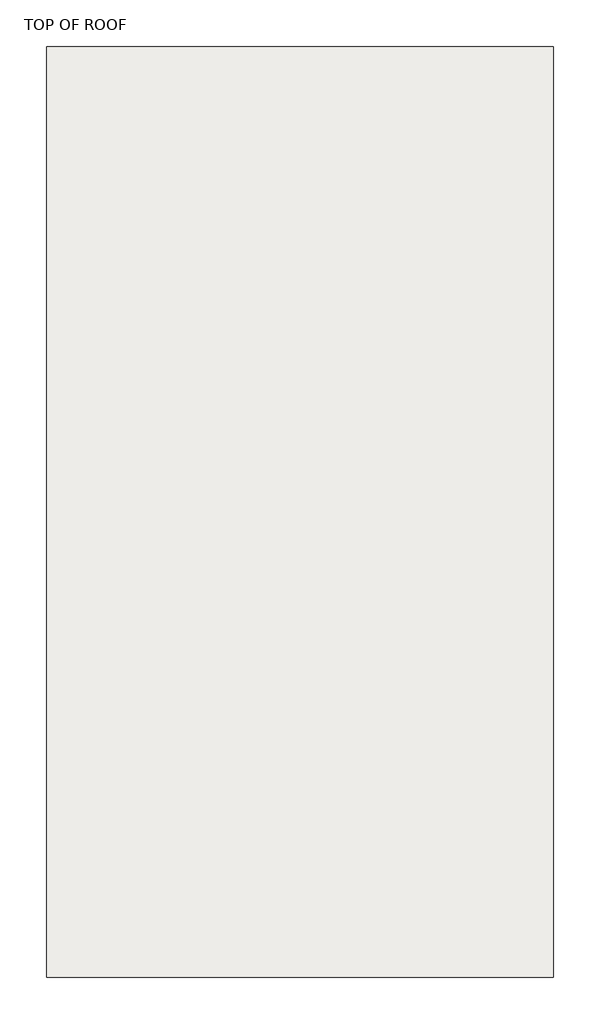
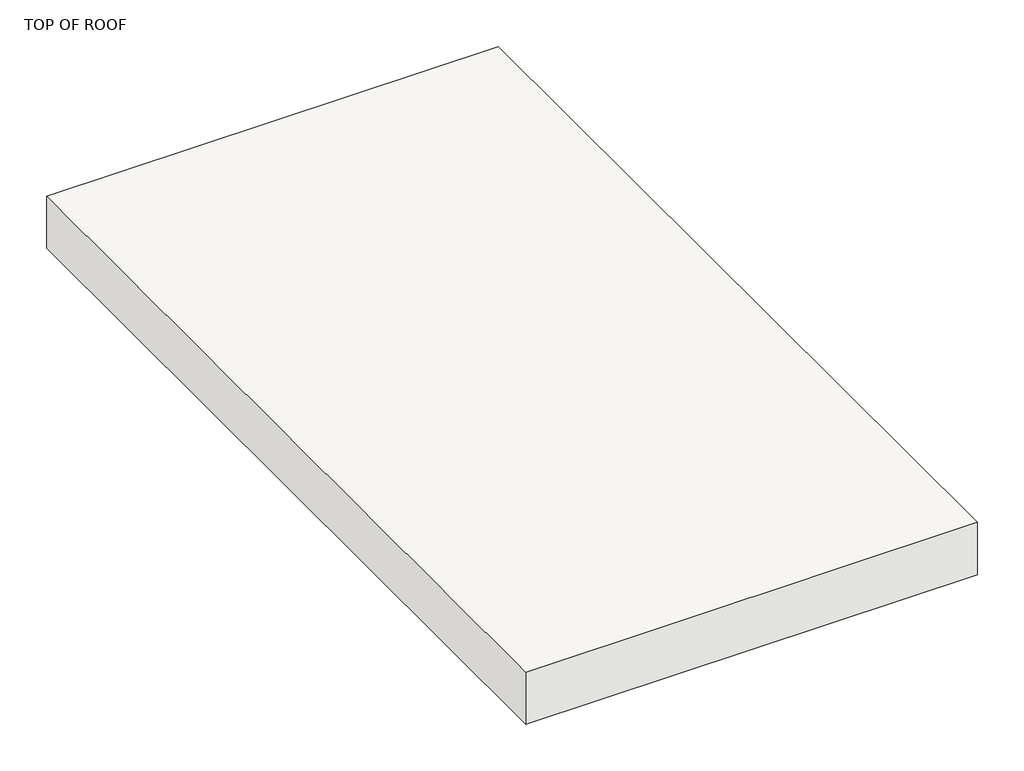
# One storey: 1 roof.
"""IFC4 building model written with IfcOpenShell, lengths in millimetres."""

from ifc_helpers import new_model, si_unit, frame, origin, place, context, project, spatial, polyline, outline, extrude, element, save

model = new_model("IFC4")

# Units and contexts
model_context = context("Model", 3, world=origin())
ifc_project = project(units=[si_unit("LENGTHUNIT", "METRE", prefix="MILLI")], contexts=[model_context])

# Site, building, storey
site = spatial("IfcSite", under=ifc_project)
building = spatial("IfcBuilding", under=site)
storey = spatial("IfcBuildingStorey", under=building, Name="TOP OF ROOF", Elevation=9144.0)

# Roof
placement = place(None, origin())
element("IfcRoof", 1, ObjectType="Generic - 12\"", at=placement, inside=storey, context=model_context, shape_type="SweptSolid", body=[
    extrude(outline(polyline([(-4757.6656154, 7090.2500875), (-2255.7656154, 7090.2500875), (-2255.7656154, 2496.7718606), (-4757.6656154, 2496.7718606), (-4757.6656154, 7090.2500875)])), frame((0.0, 0.0, 9144.0), z_axis=(0.0, 0.0, 1.0), x_axis=(1.0, 0.0, 0.0)), (0.0, 0.0, 1.0), 304.8),
])

save(model, "model.ifc")

# Revit data of these elements
# Type "Generic - 12\""
#   Assembly Code = "B1020"
#   Layers, outside or top first: 1' - 0" "Default Roof" (function 1)
# Element 1 (IfcRoof, "Generic - 12\"")
#   built-in parameter 1001705 = 31 (stored number, unit not read)
#   built-in parameter 1001710 = 33615
#   Phase Created = New Construction
#   Materials on its faces: "Default Roof"
# Materials
#   "Default Roof": colour RGB 88 101 114, transparency 0, Cost = 0
